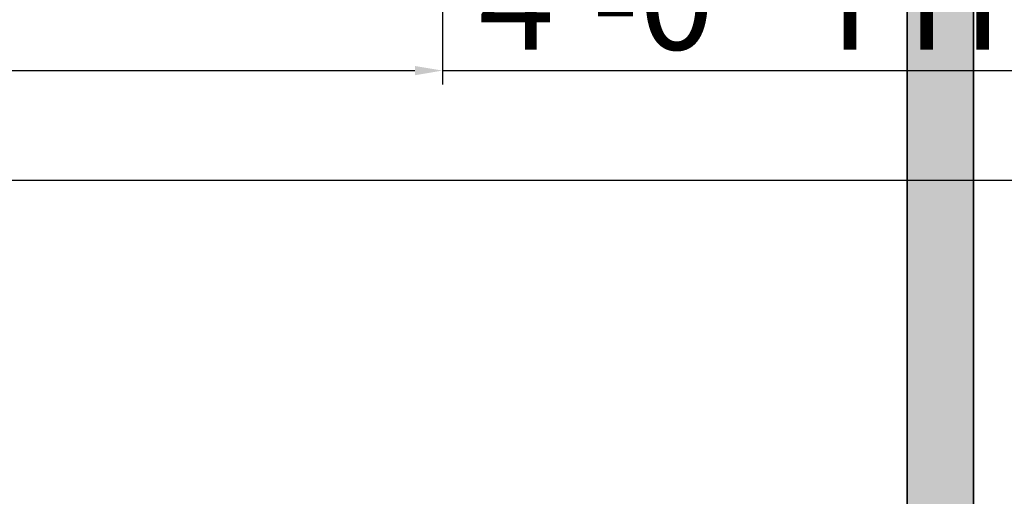
# Model space of a CAD drawing. Units: inches. Extents: x 2337 to 3570, y 1258 to 1938.
# Tile 23 of 30: x 3382 to 3471, y 1496 to 1539. Entities that reach past the tile are written whole.
import ezdxf

# ---------------------------------------------------------------- set-up
doc = ezdxf.new("R2010")
doc.units = ezdxf.units.IN
doc.layers.add('A-ANNO-DIMS', color=2, linetype='Continuous', lineweight=18)
doc.layers.add('C-PROP', color=7, linetype='Continuous', lineweight=35)
doc.layers.add('C-PROP-PATT', color=251, linetype='Continuous', lineweight=13, true_color=0x636466)
doc.styles.get("Standard").update_dxf_attribs({"font": 'arial.ttf'})
doc.dimstyles.new('ISO-25', dxfattribs={"dimtxt": 9, "dimasz": 2.5, "dimexe": 1.25, "dimexo": 0.625, "dimtad": 1, "dimdec": 1, "dimlunit": 3, "dimtxsty": 'Standard', "dimcen": 2.5, "dimadec": 0, "dimazin": 0, "dimtfac": 1, "dimtdec": 1, "dimtmove": 0, "dimatfit": 3, "dimfxl": 1, "dimarcsym": 0})

# ---------------------------------------------------------------- blocks, each defined once
blk = doc.blocks.new('*D69')
at = {"layer": 'A-ANNO-DIMS', "color": 0, "lineweight": -2, "transparency": 16777216}
for p, q in [((3371.786, 1541.491), (3371.786, 1532.766)), ((3419.786, 1541.491), (3419.786, 1532.766)), ((3374.286, 1534.016), (3417.286, 1534.016)), ((3419.786, 1534.016), (3478.758, 1534.016))]:
    blk.add_line(p, q, dxfattribs=at)
at = {"layer": 'A-ANNO-DIMS', "color": 0, "transparency": 16777216}
for points in [[(3374.286, 1534.433), (3374.286, 1533.599), (3371.786, 1534.016)], [(3417.286, 1534.433), (3417.286, 1533.599), (3419.786, 1534.016)]]:
    blk.add_solid(points, dxfattribs=at)
at = {"layer": 'Defpoints', "color": 0, "transparency": 16777216}
for p in [(3371.786, 1542.116), (3419.786, 1542.116), (3419.786, 1534.016)]:
    blk.add_point(p, dxfattribs=at)
at = {"layer": 'A-ANNO-DIMS', "color": 0, "transparency": 16777216, "insert": (3450.522, 1539.236), "char_height": 9, "attachment_point": 5}
blk.add_mtext('4\'-0" TYP.', dxfattribs=at)
blk = doc.blocks.new('*D115')
at = {"layer": 'A-ANNO-DIMS', "color": 0, "lineweight": -2, "transparency": 16777216}
for p, q in [((3243.411, 1542.116), (3502.436, 1542.116)), ((3501.186, 1539.616), (3501.186, 1526.616)), ((3243.411, 1524.116), (3502.436, 1524.116)), ((3501.186, 1524.116), (3501.186, 1497.289))]:
    blk.add_line(p, q, dxfattribs=at)
at = {"layer": 'A-ANNO-DIMS', "color": 0, "transparency": 16777216}
for points in [[(3500.769, 1539.616), (3501.603, 1539.616), (3501.186, 1542.116)], [(3500.769, 1526.616), (3501.603, 1526.616), (3501.186, 1524.116)]]:
    blk.add_solid(points, dxfattribs=at)
at = {"layer": 'Defpoints', "color": 0, "transparency": 16777216}
for p in [(3242.786, 1542.116), (3242.786, 1524.116), (3501.186, 1524.116)]:
    blk.add_point(p, dxfattribs=at)
at = {"layer": 'A-ANNO-DIMS', "color": 0, "transparency": 16777216, "insert": (3495.966, 1509.452), "char_height": 9, "attachment_point": 5, "rotation": 90}
blk.add_mtext('1\'-6"', dxfattribs=at)

msp = doc.modelspace()

# ---------------------------------------------------------------- hatches: boundary and pattern name
at = {"layer": 'C-PROP-PATT'}
h = msp.add_hatch(color=256, dxfattribs=at)
h.dxf.hatch_style = 1
h.paths.add_polyline_path([(3467.786, 1893.116), (2987.786, 1893.116), (2987.786, 1293.116), (3293.786, 1293.116), (3293.786, 1299.116), (2993.786, 1299.116), (2993.786, 1887.116), (3461.786, 1887.116), (3461.786, 1875.116), (3467.786, 1875.116)])
h.paths.add_polyline_path([(3407.786, 1299.116), (3389.786, 1299.116), (3389.786, 1293.116), (3407.786, 1293.116)], flags=17)
h.paths.add_polyline_path([(3461.786, 1299.116), (3455.786, 1299.116), (3455.786, 1293.116), (3467.786, 1293.116), (3467.786, 1779.116), (3461.786, 1779.116)], flags=17)

# ---------------------------------------------------------------- linework, layer by layer
at = {"layer": 'C-PROP'}
for p, q in [((3461.786, 1779.116), (3461.786, 1299.116)), ((3467.786, 1779.116), (3467.786, 1293.116))]:
    msp.add_line(p, q, dxfattribs=at)

# ---------------------------------------------------------------- dimensions: what is measured, and where the dimension line sits
at = {"layer": 'A-ANNO-DIMS'}
dim = msp.add_linear_dim(base=(3419.786, 1534.016), p1=(3371.786, 1542.116), p2=(3419.786, 1542.116), text='<> TYP.', dimstyle='ISO-25', override={"dimdec": 1, "dimlfac": 1, "dimrnd": 0, "dimzin": 1, "dimdsep": 46, "dimlunit": 4, "dimfrac": 2}, dxfattribs=at)
dim.commit()
dim.dimension.update_dxf_attribs({"geometry": '*D69', "text_midpoint": (3450.522, 1539.236)})
dim = msp.add_linear_dim(base=(3501.186, 1524.116), p1=(3242.786, 1542.116), p2=(3242.786, 1524.116), angle=90, dimstyle='ISO-25', override={"dimdec": 1, "dimlfac": 1, "dimrnd": 0, "dimzin": 1, "dimdsep": 46, "dimlunit": 4, "dimfrac": 2}, dxfattribs=at)
dim.commit()
dim.dimension.update_dxf_attribs({"geometry": '*D115', "text_midpoint": (3495.966, 1509.452)})

doc.saveas('drawing.dxf')
